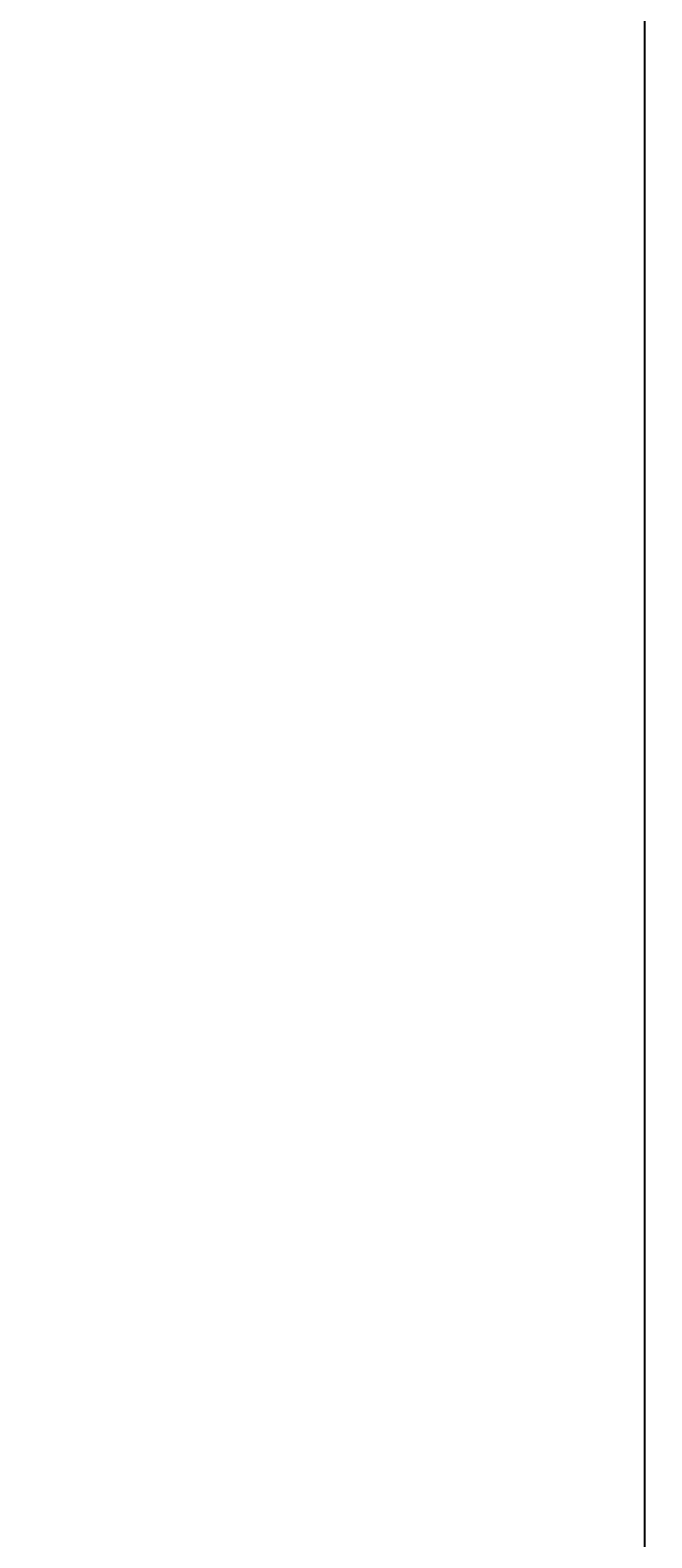
# Model space of a CAD drawing. Units: inches. Extents: x 1441 to 2460, y 1648 to 2683.
# Tile 19 of 35: x 1890 to 1916, y 2058 to 2122. Entities that reach past the tile are written whole.
import ezdxf

# ---------------------------------------------------------------- set-up
doc = ezdxf.new("R2010")
doc.units = ezdxf.units.IN
doc.layers.add('A-ANNO-DIMS', color=2, linetype='Continuous', lineweight=18)
doc.styles.get("Standard").update_dxf_attribs({"font": 'arial.ttf'})
doc.dimstyles.get("Standard").update_dxf_attribs({"dimtxt": 0.18, "dimasz": 0.18, "dimexe": 0.18, "dimexo": 0.0625, "dimgap": 0.09, "dimtad": 0, "dimtih": 1, "dimtoh": 1, "dimdec": 4, "dimzin": 0, "dimdsep": 46, "dimtxsty": 'Standard', "dimcen": 0.09, "dimadec": 0, "dimazin": 0, "dimtfac": 1, "dimtdec": 4, "dimtofl": 0, "dimtmove": 0, "dimatfit": 3, "dimfxl": 1, "dimtolj": 1, "dimtzin": 0, "dimarcsym": 0})

# ---------------------------------------------------------------- blocks, each defined once
blk = doc.blocks.new('*D67')
at = {"layer": 'A-ANNO-DIMS', "color": 0, "lineweight": -2, "transparency": 16777216}
for p, q in [((1889.448, 2298.695), (1916.216, 2298.695)), ((1916.036, 2298.515), (1916.036, 2055.938)), ((1916.036, 1812.997), (1916.036, 2055.574)), ((1758.224, 1812.817), (1916.216, 1812.817))]:
    blk.add_line(p, q, dxfattribs=at)
at = {"layer": 'A-ANNO-DIMS', "color": 0, "transparency": 16777216}
for points in [[(1916.006, 2298.515), (1916.066, 2298.515), (1916.036, 2298.695)], [(1916.006, 1812.997), (1916.066, 1812.997), (1916.036, 1812.817)]]:
    blk.add_solid(points, dxfattribs=at)
at = {"layer": 'Defpoints', "color": 0, "transparency": 16777216}
for p in [(1889.386, 2298.695), (1916.036, 2298.695), (1758.161, 1812.817)]:
    blk.add_point(p, dxfattribs=at)
at = {"layer": 'A-ANNO-DIMS', "color": 0, "transparency": 16777216, "insert": (1916.036, 2055.756), "char_height": 0.18, "attachment_point": 5}
blk.add_mtext('\\A1;485.9', dxfattribs=at)

msp = doc.modelspace()

# ---------------------------------------------------------------- dimensions: what is measured, and where the dimension line sits
at = {"layer": 'A-ANNO-DIMS'}
dim = msp.add_linear_dim(base=(1916.0359, 2298.6952), p1=(1758.1615, 1812.8171), p2=(1889.3859, 2298.6952), angle=90, dimstyle='Standard', override={"dimdec": 1, "dimlfac": 1, "dimrnd": 0, "dimzin": 0, "dimdsep": 46, "dimlunit": 2}, dxfattribs=at)
dim.commit()
dim.dimension.update_dxf_attribs({"geometry": '*D67', "text_midpoint": (1916.0359, 2055.7561)})

doc.saveas('drawing.dxf')
